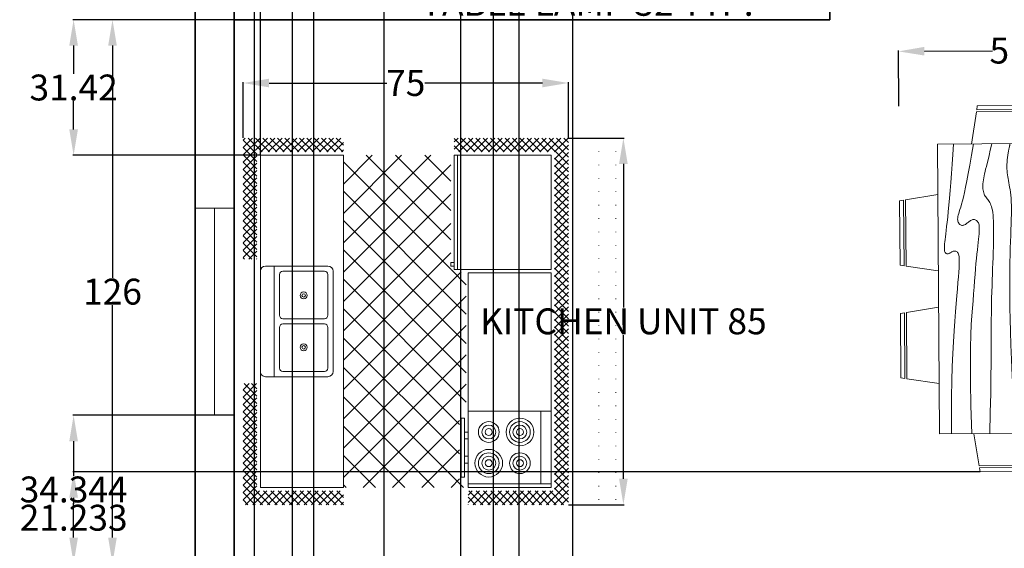
# Model space of a CAD drawing. Units: inches. Extents: x 351 to 774, y 111 to 703.
# Tile 2 of 6: x 380 to 608, y 342 to 464. Entities that reach past the tile are written whole.
import ezdxf

# ---------------------------------------------------------------- set-up
doc = ezdxf.new("R2010")
doc.units = ezdxf.units.IN
doc.header["$MEASUREMENT"] = 0
doc.linetypes.add('ACAD_ISO07W100', pattern=[3, 0, -3])
for name, color, linetype, lineweight in [('A-ANNO-DIMS', 2, 'Continuous', 18), ('A-EQPM-KTCH', 8, 'Continuous', 18), ('A-FURN', 8, 'Continuous', 18), ('A-GLAZ', 4, 'Continuous', 18), ('A-WALL', 7, 'Continuous', 35), ('A-WALL-OVHD', 7, 'ACAD_ISO07W100', 18)]:
    doc.layers.add(name, color=color, linetype=linetype, lineweight=lineweight)
doc.styles.get("Standard").update_dxf_attribs({"font": 'arial.ttf'})
doc.dimstyles.get("Standard").update_dxf_attribs({"dimtxt": 6, "dimasz": 6, "dimexe": 0.18, "dimexo": 0.0625, "dimgap": 0.09, "dimtad": 0, "dimtih": 1, "dimtoh": 1, "dimdec": 0, "dimzin": 0, "dimdsep": 46, "dimlunit": 3, "dimtxsty": 'Standard', "dimcen": 0.09, "dimadec": 0, "dimazin": 0, "dimtfac": 1, "dimtdec": 0, "dimtofl": 0, "dimtmove": 0, "dimatfit": 3, "dimfxl": 1, "dimtolj": 1, "dimtzin": 0, "dimarcsym": 0})

# ---------------------------------------------------------------- blocks, each defined once
blk = doc.blocks.new('Dining Set - 36 x 72 in.')
for p, q in [((-22, 27.5), (-22.1562, 26.50042)), ((-22, 27.5), (-6, 27.5)), ((-5.8437, 26.49966), (-6, 27.5)), ((6, 27.5), (5.8438, 26.50042)), ((6, 27.5), (22, 27.5)), ((22.1563, 26.49966), (22, 27.5)), ((-22.2343, 26.00059), (-23.4847, 17.99762)), ((-22.2304, 26), (-5.7608, 26)), ((-5.8416, 26.5), (-22.1534, 26.5)), ((-4.5152, 17.99762), (-5.7655, 25.99926)), ((5.7657, 26.00059), (4.5153, 17.99762)), ((5.7696, 26), (22.2392, 26)), ((22.1584, 26.5), (5.8466, 26.5)), ((23.4848, 17.99762), (22.2345, 25.99926)), ((36, 18), (-36, 18)), ((-36, 18), (-36, -18)), ((36, -18), (36, 18)), ((-45.5, 8), (-44.5004, 8.15617)), ((-45.5, 8), (-45.5, -8)), ((-44.5, -8.15843), (-44.5, 8.15338)), ((-44.0006, 8.23428), (-35.9976, 9.48474)), ((-44, 8.23041), (-44, -8.23915)), ((44.0006, 8.23428), (35.9976, 9.48474)), ((44, 8.23041), (44, -8.23915)), ((44.5, -8.15843), (44.5, 8.15338)), ((45.5, 8), (44.5005, 8.15617)), ((45.5, 8), (45.5, -8)), ((-44.4997, -8.15631), (-45.5, -8)), ((-35.9976, -9.48476), (-43.9993, -8.2345)), ((35.9976, -9.48476), (43.9993, -8.2345)), ((44.4997, -8.15631), (45.5, -8)), ((-36, -18), (36, -18)), ((-22.2343, -26.0006), (-23.4847, -17.99762)), ((-4.5152, -17.99762), (-5.7655, -25.99928)), ((5.7657, -26.0006), (4.5153, -17.99762)), ((23.4848, -17.99762), (22.2345, -25.99928)), ((-22.2304, -26), (-5.7608, -26)), ((-22, -27.5), (-22.1562, -26.50044)), ((-5.8416, -26.5), (-22.1534, -26.5)), ((-5.8437, -26.49967), (-6, -27.5)), ((5.7696, -26), (22.2392, -26)), ((6, -27.5), (5.8438, -26.50044)), ((22.1584, -26.5), (5.8466, -26.5)), ((22.1563, -26.49967), (22, -27.5)), ((-22, -27.5), (-6, -27.5)), ((6, -27.5), (22, -27.5))]:
    blk.add_line(p, q)
for points in [[(-36, 15), (-31.1772, 14.97754), (-26.8079, 14.91406), (-22.8538, 14.81543), (-19.276, 14.6875), (-16.0362, 14.53613), (-13.0957, 14.36718), (-10.4159, 14.18652), (-7.9583, 14), (-5.6904, 13.81315), (-3.6035, 13.63021), (-1.6954, 13.45508), (0.0365, 13.29166), (1.5945, 13.14388), (2.9811, 13.01562), (4.1988, 12.9108), (5.25, 12.83333), (6.1393, 12.78613), (6.8802, 12.76823), (7.4883, 12.77767), (7.9792, 12.8125), (8.3685, 12.87077), (8.6719, 12.95052), (8.9049, 13.0498), (9.0833, 13.16666), (9.2205, 13.29899), (9.3216, 13.44401), (9.3895, 13.59879), (9.4271, 13.76041), (9.4373, 13.92594), (9.4232, 14.09245), (9.3875, 14.257), (9.3333, 14.41666), (9.2638, 14.56917), (9.1836, 14.71484), (9.0975, 14.85465), (9.0104, 14.98958), (8.9272, 15.1206), (8.8529, 15.2487), (8.7922, 15.37483), (8.75, 15.5), (8.7305, 15.62467), (8.7344, 15.74739), (8.7617, 15.86621), (8.8125, 15.97916), (8.8867, 16.08431), (8.9844, 16.17968), (9.1055, 16.26334), (9.25, 16.33333), (9.4189, 16.38802), (9.6172, 16.42708), (9.8506, 16.45052), (10.125, 16.45833), (10.4463, 16.45052), (10.8203, 16.42708), (11.2529, 16.38802), (11.75, 16.33333), (12.3184, 16.26318), (12.9694, 16.17838), (13.7151, 16.07991), (14.5677, 15.96875), (15.5395, 15.84586), (16.6426, 15.71224), (17.8893, 15.56884), (19.2917, 15.41666), (20.859, 15.25667), (22.5879, 15.08984), (24.4721, 14.91715), (26.5052, 14.73958), (28.6809, 14.5581), (30.9929, 14.3737), (33.4347, 14.18733), (36, 14)], [(-36, 10), (-28.9766, 10.14274), (-23.1725, 10.20442), (-18.4241, 10.19775), (-14.5677, 10.13541), (-11.4399, 10.03011), (-8.877, 9.89453), (-6.7154, 9.74137), (-4.7917, 9.58333), (-2.9698, 9.43082), (-1.2246, 9.28515), (0.4415, 9.14534), (2.026, 9.01041), (3.5266, 8.87939), (4.9408, 8.7513), (6.266, 8.62516), (7.5, 8.5), (8.6411, 8.37549), (9.6914, 8.2539), (10.6538, 8.13818), (11.5312, 8.03125), (12.3267, 7.93603), (13.043, 7.85547), (13.6831, 7.79248), (14.25, 7.75), (14.7471, 7.7303), (15.1797, 7.73307), (15.5537, 7.75732), (15.875, 7.80208), (16.1494, 7.86637), (16.3828, 7.94922), (16.5811, 8.04964), (16.75, 8.16666), (16.8944, 8.29915), (17.0143, 8.44531), (17.1089, 8.60319), (17.1771, 8.77083), (17.218, 8.94629), (17.2305, 9.1276), (17.2137, 9.31282), (17.1667, 9.5), (17.0895, 9.6875), (16.987, 9.875), (16.8649, 10.0625), (16.7292, 10.25), (16.5856, 10.4375), (16.4401, 10.625), (16.2985, 10.8125), (16.1667, 11), (16.05, 11.18733), (15.9518, 11.3737), (15.8752, 11.5581), (15.8229, 11.73958), (15.798, 11.91715), (15.8034, 12.08984), (15.842, 12.25667), (15.9167, 12.41666), (16.0295, 12.56836), (16.1784, 12.70833), (16.3605, 12.83268), (16.5729, 12.9375), (16.8127, 13.01888), (17.0768, 13.07291), (17.3625, 13.0957), (17.6667, 13.08333), (17.9894, 13.03312), (18.3418, 12.94726), (18.7382, 12.82918), (19.1927, 12.68229), (19.7195, 12.51001), (20.3327, 12.31575), (21.0465, 12.10294), (21.875, 11.875), (22.8357, 11.63354), (23.959, 11.37304), (25.2786, 11.08618), (26.8282, 10.76562), (28.6414, 10.40405), (30.752, 9.99414), (33.1936, 9.52856), (36, 9)], [(-36, 5.5), (-30.7157, 5.3348), (-26.069, 5.20963), (-21.9946, 5.11767), (-18.4271, 5.05208), (-15.3009, 5.00602), (-12.5508, 4.97265), (-10.1112, 4.94515), (-7.9167, 4.91666), (-5.909, 4.88167), (-4.0586, 4.83984), (-2.3429, 4.79215), (-0.7396, 4.73958), (0.7739, 4.6831), (2.22, 4.6237), (3.6213, 4.56233), (5, 4.5), (6.373, 4.43782), (7.7344, 4.3776), (9.0723, 4.32129), (10.375, 4.27083), (11.6309, 4.22819), (12.8281, 4.19531), (13.9551, 4.17415), (15, 4.16666), (15.954, 4.17448), (16.819, 4.19791), (17.6001, 4.23698), (18.3021, 4.29166), (18.9299, 4.36198), (19.4883, 4.44791), (19.9823, 4.54948), (20.4167, 4.66666), (20.7969, 4.79899), (21.1302, 4.94401), (21.4245, 5.09879), (21.6875, 5.26041), (21.9271, 5.42594), (22.1511, 5.59245), (22.3672, 5.757), (22.5834, 5.91666), (22.8065, 6.06868), (23.0404, 6.21093), (23.2879, 6.34147), (23.5521, 6.45833), (23.8358, 6.55957), (24.142, 6.64323), (24.4735, 6.70735), (24.8334, 6.75), (25.2235, 6.76969), (25.642, 6.76692), (26.0858, 6.74267), (26.5521, 6.69791), (27.0379, 6.63362), (27.5404, 6.55078), (28.0565, 6.45036), (28.5834, 6.33333), (29.1242, 6.19987), (29.7071, 6.04687), (30.3661, 5.87044), (31.1354, 5.66666), (32.0493, 5.43164), (33.142, 5.16146), (34.4475, 4.85221), (36, 4.5)], [(-36, -1), (-30.7915, -0.6591), (-26.0195, -0.38216), (-21.6519, -0.16284), (-17.6563, 0.00521), (-14.0005, 0.12833), (-10.6523, 0.21289), (-7.5796, 0.26522), (-4.75, 0.29166), (-2.134, 0.29793), (0.2878, 0.28711), (2.5317, 0.26163), (4.6146, 0.22396), (6.5529, 0.17651), (8.3633, 0.12174), (10.0623, 0.06209), (11.6667, 0), (13.1899, -0.06201), (14.6341, -0.1211), (15.9982, -0.17432), (17.2813, -0.21875), (18.4823, -0.25147), (19.6003, -0.26953), (20.6343, -0.27002), (21.5834, -0.25), (22.4481, -0.20768), (23.2357, -0.14584), (23.9549, -0.06836), (24.6146, 0.02083), (25.2235, 0.11784), (25.7904, 0.21875), (26.3241, 0.31966), (26.8334, 0.41666), (27.3265, 0.50618), (27.8099, 0.58593), (28.2894, 0.65397), (28.7709, 0.70833), (29.2601, 0.74707), (29.763, 0.76823), (30.2855, 0.76985), (30.8334, 0.75), (31.4088, 0.70784), (31.9994, 0.64713), (32.589, 0.57275), (33.1615, 0.48958), (33.7008, 0.4025), (34.1908, 0.3164), (34.6153, 0.23616), (34.9584, 0.16666), (35.2099, 0.11165), (35.3848, 0.07031), (35.504, 0.04069), (35.5886, 0.02083), (35.6594, 0.00879), (35.7377, 0.0026), (35.8442, 0.00032), (36, 0)], [(-36, -6.5), (-27.1843, -6.31267), (-20.084, -6.1263), (-14.469, -5.9419), (-10.1094, -5.76042), (-6.7752, -5.58285), (-4.2363, -5.41016), (-2.2629, -5.24333), (-0.625, -5.08334), (0.8708, -4.93099), (2.2715, -4.78646), (3.5872, -4.64974), (4.8281, -4.52084), (6.0046, -4.39974), (7.127, -4.28646), (8.2053, -4.18099), (9.25, -4.08334), (10.2705, -3.99382), (11.2734, -3.91407), (12.2647, -3.84603), (13.25, -3.79167), (14.2354, -3.75293), (15.2266, -3.73177), (16.2295, -3.73015), (17.25, -3.75), (18.2912, -3.79248), (19.3451, -3.85547), (20.4009, -3.93604), (21.4479, -4.03125), (22.4754, -4.13819), (23.4727, -4.25391), (24.4289, -4.37549), (25.3334, -4.5), (26.1785, -4.62492), (26.9694, -4.74935), (27.7145, -4.87281), (28.4219, -4.99479), (29.1, -5.11483), (29.7572, -5.23242), (30.4016, -5.34709), (31.0417, -5.45834), (31.6837, -5.56437), (32.3262, -5.65821), (32.9658, -5.73153), (33.599, -5.77604), (34.2224, -5.78345), (34.8327, -5.74545), (35.4264, -5.65373), (36, -5.5)], [(-36, -10), (-26.4022, -9.81299), (-18.4675, -9.62891), (-11.9839, -9.45069), (-6.7396, -9.28125), (-2.5226, -9.12354), (0.8789, -8.98047), (3.6769, -8.85498), (6.0833, -8.75), (8.2767, -8.66765), (10.3021, -8.60677), (12.1712, -8.56543), (13.8958, -8.54167), (15.4876, -8.53353), (16.9583, -8.53907), (18.3197, -8.55632), (19.5834, -8.58334), (20.7616, -8.61841), (21.8685, -8.66081), (22.9188, -8.71004), (23.9271, -8.76563), (24.9081, -8.82707), (25.8763, -8.89388), (26.8465, -8.96558), (27.8334, -9.04167), (28.8474, -9.12118), (29.8828, -9.20117), (30.93, -9.27824), (31.9792, -9.34896), (33.0205, -9.40991), (34.0443, -9.45768), (35.0407, -9.48885), (36, -9.5)], [(-36, -14.5), (-30.0881, -14.33513), (-25.0332, -14.21224), (-20.7312, -14.12647), (-17.0781, -14.07292), (-13.97, -14.04671), (-11.3027, -14.04297), (-8.9724, -14.05681), (-6.875, -14.08334), (-4.9224, -14.11833), (-3.0905, -14.16016), (-1.3709, -14.20785), (0.2448, -14.26042), (1.7647, -14.3169), (3.1973, -14.3763), (4.5507, -14.43767), (5.8333, -14.5), (7.0554, -14.5621), (8.235, -14.62175), (9.3922, -14.67652), (10.5469, -14.72396), (11.7192, -14.76164), (12.929, -14.78711), (14.1965, -14.79794), (15.5417, -14.79167), (16.9933, -14.76424), (18.6152, -14.70508), (20.4804, -14.60197), (22.6615, -14.44271), (25.2312, -14.21509), (28.2624, -13.9069), (31.8277, -13.50594), (36, -13)]]:
    blk.add_lwpolyline(points)
blk = doc.blocks.new('Kitchen Layout - 7 x 8 ft')
for p, q in [((-5, 81.32), (2.68, 89)), ((-5, 83.44), (0.56, 89)), ((-5, 85.56), (-1.56, 89)), ((-5, 87.68), (-3.68, 89)), ((-1, 84.97), (-5, 88.97)), ((1.09, 85), (-2.91, 89)), ((3.21, 85), (-0.79, 89)), ((0.81, 85), (4.81, 89)), ((5.34, 85), (1.34, 89)), ((2.93, 85), (6.93, 89)), ((7.46, 85), (3.46, 89)), ((5.05, 85), (9.05, 89)), ((9.58, 85), (5.58, 89)), ((7.17, 85), (11.17, 89)), ((11.7, 85), (7.7, 89)), ((9.29, 85), (13.29, 89)), ((13.82, 85), (9.82, 89)), ((11.41, 85), (15.41, 89)), ((15.94, 85), (11.94, 89)), ((13.53, 85), (17.53, 89)), ((18.06, 85), (14.06, 89)), ((15.65, 85), (19.65, 89)), ((20.18, 85), (16.18, 89)), ((17.78, 85), (21.78, 89)), ((22.31, 85), (18.31, 89)), ((19.9, 85), (23.9, 89)), ((24.43, 85), (20.43, 89)), ((22.02, 85), (26.02, 89)), ((26.55, 85), (22.55, 89)), ((24.14, 85), (28.14, 89)), ((28.67, 85), (24.67, 89)), ((26.26, 85), (30.26, 89)), ((30.79, 85), (26.79, 89)), ((28.38, 85), (32.38, 89)), ((32.91, 85), (28.91, 89)), ((30.5, 85), (34.5, 89)), ((35.03, 85), (31.03, 89)), ((32.63, 85), (36.63, 89)), ((37.16, 85), (33.16, 89)), ((34.75, 85), (38.75, 89)), ((39.28, 85), (35.28, 89)), ((36.87, 85), (40.87, 89)), ((41.4, 85), (37.4, 89)), ((38.99, 85), (42.99, 89)), ((43.52, 85), (39.52, 89)), ((41.11, 85), (45.11, 89)), ((45.64, 85), (41.64, 89)), ((43.23, 85), (47.23, 89)), ((47.76, 85), (43.76, 89)), ((45.35, 85), (49.35, 89)), ((49.88, 85), (45.88, 89)), ((47.47, 85), (51.47, 89)), ((52, 85), (48, 89)), ((49.6, 85), (53.6, 89)), ((54.13, 85), (50.13, 89)), ((51.72, 85), (55.72, 89)), ((56.25, 85), (52.25, 89)), ((53.84, 85), (57.84, 89)), ((58.37, 85), (54.37, 89)), ((55.96, 85), (59.96, 89)), ((60.49, 85), (56.49, 89)), ((58.08, 85), (62.08, 89)), ((62.61, 85), (58.61, 89)), ((60.2, 85), (64.2, 89)), ((64.73, 85), (60.73, 89)), ((62.32, 85), (66.32, 89)), ((66.85, 85), (62.85, 89)), ((64.45, 85), (68.45, 89)), ((68.97, 85), (64.97, 89)), ((66.57, 85), (70.57, 89)), ((71.1, 85), (67.1, 89)), ((68.69, 85), (72.69, 89)), ((73.22, 85), (69.22, 89)), ((70.81, 85), (74.81, 89)), ((75.34, 85), (71.34, 89)), ((72.93, 85), (76.93, 89)), ((77.46, 85), (73.46, 89)), ((75.05, 85), (79.05, 89)), ((79.58, 85), (75.58, 89)), ((77.17, 85), (81.17, 89)), ((81.7, 85), (77.7, 89)), ((79.29, 85), (83.29, 89)), ((83.82, 85), (79.82, 89)), ((81.42, 85), (85.42, 89)), ((85.95, 85), (81.95, 89)), ((83.54, 85), (87.54, 89)), ((88.07, 85), (84.07, 89)), ((85.66, 85), (89.66, 89)), ((90.19, 85), (86.19, 89)), ((87.78, 85), (91.78, 89)), ((92.31, 85), (88.31, 89)), ((89.9, 85), (93.9, 89)), ((94.43, 85), (90.43, 89)), ((92.02, 85), (96.02, 89)), ((96.55, 85), (92.55, 89)), ((94.14, 85), (98.14, 89)), ((101, 82.67), (94.67, 89)), ((96.27, 85), (100.27, 89)), ((101, 84.79), (96.79, 89)), ((101, 86.92), (98.92, 89)), ((-1, 82.85), (-5, 86.85)), ((97, 83.61), (101, 87.61)), ((97, 81.49), (101, 85.49)), ((-1, 80.73), (-5, 84.73)), ((-5, 79.19), (-1, 83.19)), ((-1, 78.61), (-5, 82.61)), ((34, 84), (96, 84)), ((34, 60), (34, 84)), ((96, 84), (96, 60)), ((101, 80.55), (97, 84.55)), ((97, 79.37), (101, 83.37)), ((-5, 77.07), (-1, 81.07)), ((-1, 76.49), (-5, 80.49)), ((74, 81), (95, 81)), ((101, 78.43), (97, 82.43)), ((97, 77.25), (101, 81.25)), ((101, 76.31), (97, 80.31)), ((-5, 74.95), (-1, 78.95)), ((-1, 74.36), (-5, 78.36)), ((97, 75.13), (101, 79.13)), ((101, 74.19), (97, 78.19)), ((97, 73.01), (101, 77.01)), ((-5, 72.83), (-1, 76.83)), ((-1, 72.24), (-5, 76.24)), ((-5, 70.71), (-1, 74.71)), ((-1, 70.12), (-5, 74.12)), ((101, 72.07), (97, 76.07)), ((97, 70.89), (101, 74.89)), ((-5, 68.59), (-1, 72.59)), ((-1, 68), (-5, 72)), ((101, 69.95), (97, 73.95)), ((97, 68.76), (101, 72.76)), ((101, 67.82), (97, 71.82)), ((-5, 66.47), (-1, 70.47)), ((-1, 65.88), (-5, 69.88)), ((-5, 64.35), (-1, 68.35)), ((97, 66.64), (101, 70.64)), ((101, 65.7), (97, 69.7)), ((97, 64.52), (101, 68.52)), ((-1, 63.76), (-5, 67.76)), ((-5, 62.22), (-1, 66.22)), ((-1, 61.64), (-5, 65.64)), ((101, 63.58), (97, 67.58)), ((97, 62.4), (101, 66.4)), ((101, 61.46), (97, 65.46)), ((-5, 60.1), (-1, 64.1)), ((-1, 59.52), (-5, 63.52)), ((97, 60.28), (101, 64.28)), ((100.34, 60), (97, 63.34)), ((-5, 57.98), (-1, 61.98)), ((-1, 57.39), (-5, 61.39)), ((-4.86, 56), (-1, 59.86)), ((96, 60), (34, 60)), ((80, 60), (80, 59)), ((82, 59), (82, 60)), ((87, 59), (87, 60)), ((89, 60), (89, 59)), ((98.22, 60), (97, 61.22)), ((98.84, 60), (101, 62.16)), ((100.96, 60), (101, 60.04)), ((-1.73, 56), (-5, 59.27)), ((-3.85, 56), (-5, 57.15)), ((-2.74, 56), (-1, 57.74)), ((0, 57), (33, 57)), ((10.4, 24), (45.9, 59.5)), ((18.88, 24), (54.38, 59.5)), ((27.37, 24), (62.87, 59.5)), ((33.03, 55.11), (37.41, 59.5)), ((67.71, 24), (33.68, 58.04)), ((35.85, 24), (71.35, 59.5)), ((76.2, 24), (40.7, 59.5)), ((44.34, 24), (77.84, 57.5)), ((84.68, 24), (49.18, 59.5)), ((52.82, 24), (86.32, 57.5)), ((93.17, 24), (57.67, 59.5)), ((61.31, 24), (96, 58.69)), ((96, 29.65), (66.15, 59.5)), ((96, 38.14), (76.64, 57.5)), ((96, 46.63), (85.13, 57.5)), ((96, 55.11), (93.57, 57.54)), ((0, 30.57), (24.43, 55)), ((0, 39.06), (15.94, 55)), ((0, 47.54), (7.46, 55)), ((1.91, 24), (32.91, 55)), ((33.77, 24), (2.77, 55)), ((42.26, 24), (11.26, 55)), ((50.74, 24), (19.74, 55)), ((59.23, 24), (28.23, 55)), ((31, 55), (31, 56)), ((32, 55), (31, 55)), ((32, 56), (32, 55)), ((25.29, 24), (0, 49.29)), ((69.79, 24), (96, 50.21)), ((16.8, 24), (0, 40.8)), ((78.28, 24), (96, 41.72)), ((8.32, 24), (0, 32.32)), ((86.76, 24), (96, 33.24)), ((-5, 21.92), (-2.92, 24)), ((-5, 19.8), (-1, 23.8)), ((-1, 19.21), (-5, 23.21)), ((-1, 21.33), (-3.67, 24)), ((-1, 23.45), (-1.55, 24)), ((0, 24), (96, 24)), ((0, 0), (0, 24)), ((95.25, 24), (96, 24.75)), ((96, 24), (96, 0)), ((97, 22.1), (98.9, 24)), ((97, 19.97), (101, 23.97)), ((101, 19.03), (97, 23.03)), ((101, 21.16), (98.16, 24)), ((101, 23.28), (100.28, 24)), ((-5, 17.68), (-1, 21.68)), ((-1, 17.09), (-5, 21.09)), ((97, 17.85), (101, 21.85)), ((101, 16.91), (97, 20.91)), ((-5, 15.55), (-1, 19.55)), ((-1, 14.97), (-5, 18.97)), ((-5, 13.43), (-1, 17.43)), ((47.25, 6.5), (47.25, 18.5)), ((48.75, 18.5), (48.75, 6.5)), ((97, 15.73), (101, 19.73)), ((101, 14.79), (97, 18.79)), ((97, 13.61), (101, 17.61)), ((-1, 12.85), (-5, 16.85)), ((-5, 11.31), (-1, 15.31)), ((-1, 10.73), (-5, 14.73)), ((101, 12.67), (97, 16.67)), ((97, 11.49), (101, 15.49)), ((101, 10.55), (97, 14.55)), ((-5, 9.19), (-1, 13.19)), ((-1, 8.6), (-5, 12.6)), ((97, 9.37), (101, 13.37)), ((101, 8.43), (97, 12.43)), ((-5, 7.07), (-1, 11.07)), ((-1, 6.48), (-5, 10.48)), ((-5, 4.95), (-1, 8.95)), ((97, 7.25), (101, 11.25)), ((101, 6.31), (97, 10.31)), ((97, 5.12), (101, 9.12)), ((-1, 4.36), (-5, 8.36)), ((-5, 2.83), (-1, 6.83)), ((-1, 2.24), (-5, 6.24)), ((101, 4.18), (97, 8.18)), ((97, 3), (101, 7)), ((101, 2.06), (97, 6.06)), ((-5, 0.71), (-1, 4.71)), ((-1, 0.12), (-5, 4.12)), ((64, 4), (32, 4)), ((97, 0.88), (101, 4.88)), ((101, -0.06), (97, 3.94)), ((-5, -1.42), (-1, 2.58)), ((2, -5), (-5, 2)), ((-5, -3.54), (-1, 0.46)), ((96, 0), (0, 0)), ((93.24, -5), (101, 2.76)), ((95.36, -5), (101, 0.64)), ((101, -2.18), (97, 1.82)), ((-0.12, -5), (-5, -0.12)), ((-2.25, -5), (-5, -2.25)), ((-4.34, -5), (-0.34, -1)), ((-2.22, -5), (1.78, -1)), ((-0.1, -5), (3.9, -1)), ((4.12, -5), (0.12, -1)), ((2.02, -5), (6.02, -1)), ((6.24, -5), (2.24, -1)), ((4.14, -5), (8.14, -1)), ((8.36, -5), (4.36, -1)), ((6.27, -5), (10.27, -1)), ((10.48, -5), (6.48, -1)), ((8.39, -5), (12.39, -1)), ((12.6, -5), (8.6, -1)), ((10.51, -5), (14.51, -1)), ((14.73, -5), (10.73, -1)), ((12.63, -5), (16.63, -1)), ((16.85, -5), (12.85, -1)), ((14.75, -5), (18.75, -1)), ((18.97, -5), (14.97, -1)), ((16.87, -5), (20.87, -1)), ((21.09, -5), (17.09, -1)), ((18.99, -5), (22.99, -1)), ((23.21, -5), (19.21, -1)), ((21.11, -5), (25.11, -1)), ((25.33, -5), (21.33, -1)), ((23.24, -5), (27.24, -1)), ((27.45, -5), (23.45, -1)), ((25.36, -5), (29.36, -1)), ((29.57, -5), (25.57, -1)), ((27.48, -5), (30, -2.48)), ((30, -3.3), (27.7, -1)), ((30, -1.18), (29.82, -1)), ((66, -2.54), (67.54, -1)), ((66, -4.66), (69.66, -1)), ((69.88, -5), (66, -1.12)), ((67.78, -5), (71.78, -1)), ((72, -5), (68, -1)), ((69.9, -5), (73.9, -1)), ((74.12, -5), (70.12, -1)), ((72.03, -5), (76.03, -1)), ((76.24, -5), (72.24, -1)), ((74.15, -5), (78.15, -1)), ((78.36, -5), (74.36, -1)), ((76.27, -5), (80.27, -1)), ((80.49, -5), (76.49, -1)), ((78.39, -5), (82.39, -1)), ((82.61, -5), (78.61, -1)), ((80.51, -5), (84.51, -1)), ((84.73, -5), (80.73, -1)), ((82.63, -5), (86.63, -1)), ((86.85, -5), (82.85, -1)), ((84.75, -5), (88.75, -1)), ((88.97, -5), (84.97, -1)), ((86.88, -5), (90.88, -1)), ((91.09, -5), (87.09, -1)), ((89, -5), (93, -1)), ((93.21, -5), (89.21, -1)), ((91.12, -5), (95.12, -1)), ((95.34, -5), (91.34, -1)), ((97.46, -5), (93.46, -1)), ((99.58, -5), (95.58, -1)), ((101, -4.3), (97, -0.3)), ((97.48, -5), (101, -1.48)), ((-4.37, -5), (-5, -4.37)), ((29.6, -5), (30, -4.6)), ((67.76, -5), (66, -3.24)), ((99.6, -5), (101, -3.6))]:
    blk.add_line(p, q)
for points in [[(0, 56), (0, 84), (33, 84), (33, 56)], [(74, 60), (74, 84), (95, 84), (95, 60)], [(76, 58), (76, 59), (93, 59), (93, 58)]]:
    blk.add_lwpolyline(points, close=True)
for points in [[(33.5, 21), (62.5, 21)], [(32, 1.5), (32, 19.5)], [(33.5, 6.5), (33.5, 18.5)], [(34.5, 19.5), (46.25, 19.5)], [(49.75, 19.5), (61.5, 19.5)], [(62.5, 18.5), (62.5, 6.5)], [(64, 19.5), (64, 1.5)], [(46.25, 5.5), (34.5, 5.5)], [(61.5, 5.5), (49.75, 5.5)], [(62.5, 0), (33.5, 0)]]:
    blk.add_lwpolyline(points)
for centre, radius in [((80, 75), 4), ((80, 75), 3), ((80, 75), 2), ((89, 75), 3), ((89, 75), 2), ((80, 75), 1), ((89, 75), 1), ((80, 66), 3), ((89, 66), 4), ((89, 66), 3), ((80, 66), 2), ((80, 66), 1), ((89, 66), 2), ((89, 66), 1), ((40.5, 12.5), 1), ((40.5, 12.5), 0.5), ((55.5, 12.5), 1), ((55.5, 12.5), 0.5)]:
    blk.add_circle(centre, radius)
for centre, radius, start, end in [((33.5, 19.5), 1.5, 90, 180), ((62.5, 19.5), 1.5, 0, 90), ((34.5, 18.5), 1, 90, 180), ((46.25, 18.5), 1, 0, 90), ((49.75, 18.5), 1, 90, 180), ((61.5, 18.5), 1, 0, 90), ((34.5, 6.5), 1, 180, 270), ((46.25, 6.5), 1, 270, 0), ((49.75, 6.5), 1, 180, 270), ((61.5, 6.5), 1, 270, 0), ((33.5, 1.5), 1.5, 180, 270), ((62.5, 1.5), 1.5, 270, 0)]:
    blk.add_arc(centre, radius, start, end)
blk = doc.blocks.new('WIN-48IN-9IN-WALL')
blk.add_line((4.5, 48), (4.5, 0))
blk.add_lwpolyline([(0, 0), (9, 0), (9, 48), (0, 48)], close=True)
blk = doc.blocks.new('*D28')
at = {"layer": 'A-ANNO-DIMS', "color": 0, "lineweight": -2, "transparency": 16777216}
for p, q in [((432.23, 472.86), (432.23, 467.97)), ((464.06, 472.86), (464.06, 467.97)), ((438.23, 468.15), (458.06, 468.15)), ((464.06, 468.15), (470.06, 468.15))]:
    blk.add_line(p, q, dxfattribs=at)
at = {"layer": 'A-ANNO-DIMS', "color": 0, "transparency": 16777216}
for points in [[(438.23, 469.15), (438.23, 467.15), (432.23, 468.15)], [(458.06, 469.15), (458.06, 467.15), (464.06, 468.15)]]:
    blk.add_solid(points, dxfattribs=at)
at = {"layer": 'Defpoints', "color": 0, "transparency": 16777216}
for p in [(432.23, 472.92), (464.06, 472.92), (464.06, 468.15)]:
    blk.add_point(p, dxfattribs=at)
at = {"layer": 'A-ANNO-DIMS', "color": 0, "transparency": 16777216, "insert": (511.85, 468.15), "char_height": 6, "attachment_point": 5}
blk.add_mtext('\\A1;TABLE LAMP 32 TYP.', dxfattribs=at)
blk = doc.blocks.new('*D37')
at = {"layer": 'A-ANNO-DIMS', "color": 0, "lineweight": -2, "transparency": 16777216}
for p, q in [((584.02, 444.23), (583.93, 457.08)), ((589.93, 456.94), (605.75, 457.06)), ((629.2, 457.23), (613.37, 457.11)), ((635.29, 444.61), (635.2, 457.45))]:
    blk.add_line(p, q, dxfattribs=at)
at = {"layer": 'A-ANNO-DIMS', "color": 0, "transparency": 16777216}
for points in [[(589.92, 457.94), (589.93, 455.94), (583.93, 456.9)], [(629.19, 458.23), (629.21, 456.23), (635.2, 457.27)]]:
    blk.add_solid(points, dxfattribs=at)
at = {"layer": 'Defpoints', "color": 0, "transparency": 16777216}
for p in [(583.93, 456.9), (584.02, 444.17), (635.29, 444.55)]:
    blk.add_point(p, dxfattribs=at)
at = {"layer": 'A-ANNO-DIMS', "color": 0, "transparency": 16777216, "insert": (609.56, 457.08), "char_height": 6, "attachment_point": 5}
blk.add_mtext('\\A1;51', dxfattribs=at)
blk = doc.blocks.new('*D44')
at = {"layer": 'A-ANNO-DIMS', "color": 0, "lineweight": -2, "transparency": 16777216}
for p, q in [((507.54, 436.83), (520.4, 436.83)), ((520.22, 430.83), (520.22, 397.55)), ((520.22, 357.88), (520.22, 391.16)), ((507.54, 351.88), (520.4, 351.88))]:
    blk.add_line(p, q, dxfattribs=at)
at = {"layer": 'A-ANNO-DIMS', "color": 0, "transparency": 16777216}
for points in [[(519.22, 430.83), (521.22, 430.83), (520.22, 436.83)], [(519.22, 357.88), (521.22, 357.88), (520.22, 351.88)]]:
    blk.add_solid(points, dxfattribs=at)
at = {"layer": 'Defpoints', "color": 0, "transparency": 16777216}
for p in [(507.48, 436.83), (507.48, 351.88), (520.22, 351.88)]:
    blk.add_point(p, dxfattribs=at)
at = {"layer": 'A-ANNO-DIMS', "color": 0, "transparency": 16777216, "insert": (520.22, 394.36), "char_height": 6, "attachment_point": 5}
blk.add_mtext('\\A1;KITCHEN UNIT 85', dxfattribs=at)
blk = doc.blocks.new('*D45')
at = {"layer": 'A-ANNO-DIMS', "color": 0, "lineweight": -2, "transparency": 16777216}
for p, q in [((432.15, 436.89), (432.15, 449.75)), ((438.15, 449.57), (465.43, 449.57)), ((501.48, 449.57), (474.2, 449.57)), ((507.48, 436.89), (507.48, 449.75))]:
    blk.add_line(p, q, dxfattribs=at)
at = {"layer": 'A-ANNO-DIMS', "color": 0, "transparency": 16777216}
for points in [[(438.15, 450.57), (438.15, 448.57), (432.15, 449.57)], [(501.48, 450.57), (501.48, 448.57), (507.48, 449.57)]]:
    blk.add_solid(points, dxfattribs=at)
at = {"layer": 'Defpoints', "color": 0, "transparency": 16777216}
for p in [(507.48, 449.57), (432.15, 436.83), (507.48, 436.83)]:
    blk.add_point(p, dxfattribs=at)
at = {"layer": 'A-ANNO-DIMS', "color": 0, "transparency": 16777216, "insert": (469.81, 449.57), "char_height": 6, "attachment_point": 5}
blk.add_mtext('\\A1;75', dxfattribs=at)
blk = doc.blocks.new('*D50')
at = {"layer": 'A-ANNO-DIMS', "color": 0, "lineweight": -2, "transparency": 16777216}
for p, q in [((421.04, 671.18), (421.04, 114.91)), ((443.48, 671.18), (443.48, 114.91)), ((427.04, 115.09), (437.48, 115.09)), ((443.48, 115.09), (449.48, 115.09))]:
    blk.add_line(p, q, dxfattribs=at)
at = {"layer": 'A-ANNO-DIMS', "color": 0, "transparency": 16777216}
for points in [[(427.04, 116.09), (427.04, 114.09), (421.04, 115.09)], [(437.48, 116.09), (437.48, 114.09), (443.48, 115.09)]]:
    blk.add_solid(points, dxfattribs=at)
at = {"layer": 'Defpoints', "color": 0, "transparency": 16777216}
for p in [(421.04, 671.24), (443.48, 671.24), (443.48, 115.09)]:
    blk.add_point(p, dxfattribs=at)
at = {"layer": 'A-ANNO-DIMS', "color": 0, "transparency": 16777216, "insert": (462.06, 115.09), "char_height": 6, "attachment_point": 5}
blk.add_mtext('\\A1;22.434', dxfattribs=at)
blk = doc.blocks.new('*D55')
at = {"layer": 'A-ANNO-DIMS', "color": 0, "lineweight": -2, "transparency": 16777216}
for p, q in [((429.98, 372.59), (392.71, 372.59)), ((392.89, 366.59), (392.89, 358.57)), ((392.89, 344.24), (392.89, 352.26)), ((429.98, 338.24), (392.71, 338.24))]:
    blk.add_line(p, q, dxfattribs=at)
at = {"layer": 'A-ANNO-DIMS', "color": 0, "transparency": 16777216}
for points in [[(391.89, 366.59), (393.89, 366.59), (392.89, 372.59)], [(391.89, 344.24), (393.89, 344.24), (392.89, 338.24)]]:
    blk.add_solid(points, dxfattribs=at)
at = {"layer": 'Defpoints', "color": 0, "transparency": 16777216}
for p in [(392.89, 372.59), (430.04, 372.59), (430.04, 338.24)]:
    blk.add_point(p, dxfattribs=at)
at = {"layer": 'A-ANNO-DIMS', "color": 0, "transparency": 16777216, "insert": (392.89, 355.41), "char_height": 6, "attachment_point": 5}
blk.add_mtext('\\A1;34.344', dxfattribs=at)
blk = doc.blocks.new('*D56')
at = {"layer": 'A-ANNO-DIMS', "color": 0, "lineweight": -2, "transparency": 16777216}
for p, q in [((429.98, 464.24), (401.71, 464.24)), ((401.89, 458.24), (401.89, 404.4)), ((401.89, 344.24), (401.89, 398.09)), ((429.98, 338.24), (401.71, 338.24))]:
    blk.add_line(p, q, dxfattribs=at)
at = {"layer": 'A-ANNO-DIMS', "color": 0, "transparency": 16777216}
for points in [[(400.89, 458.24), (402.89, 458.24), (401.89, 464.24)], [(400.89, 344.24), (402.89, 344.24), (401.89, 338.24)]]:
    blk.add_solid(points, dxfattribs=at)
at = {"layer": 'Defpoints', "color": 0, "transparency": 16777216}
for p in [(401.89, 464.24), (430.04, 464.24), (430.04, 338.24)]:
    blk.add_point(p, dxfattribs=at)
at = {"layer": 'A-ANNO-DIMS', "color": 0, "transparency": 16777216, "insert": (401.89, 401.24), "char_height": 6, "attachment_point": 5}
blk.add_mtext('\\A1;126', dxfattribs=at)
blk = doc.blocks.new('*D70')
at = {"layer": 'A-ANNO-DIMS', "color": 0, "lineweight": -2, "transparency": 16777216}
for p, q in [((430.04, 614.18), (430.04, 114.91)), ((434.71, 614.18), (434.71, 114.91)), ((424.04, 115.09), (418.04, 115.09)), ((440.71, 115.09), (446.71, 115.09))]:
    blk.add_line(p, q, dxfattribs=at)
at = {"layer": 'A-ANNO-DIMS', "color": 0, "transparency": 16777216}
for points in [[(424.04, 116.09), (424.04, 114.09), (430.04, 115.09)], [(440.71, 116.09), (440.71, 114.09), (434.71, 115.09)]]:
    blk.add_solid(points, dxfattribs=at)
at = {"layer": 'Defpoints', "color": 0, "transparency": 16777216}
for p in [(430.04, 614.24), (434.71, 614.24), (434.71, 115.09)]:
    blk.add_point(p, dxfattribs=at)
at = {"layer": 'A-ANNO-DIMS', "color": 0, "transparency": 16777216, "insert": (457.05, 115.09), "char_height": 6, "attachment_point": 5}
blk.add_mtext('\\A1;4.669', dxfattribs=at)
blk = doc.blocks.new('*D71')
at = {"layer": 'A-ANNO-DIMS', "color": 0, "lineweight": -2, "transparency": 16777216}
for p, q in [((434.71, 614.18), (434.71, 114.91)), ((464.71, 614.18), (464.71, 114.91)), ((440.71, 115.09), (445.34, 115.09)), ((458.71, 115.09), (454.09, 115.09))]:
    blk.add_line(p, q, dxfattribs=at)
at = {"layer": 'A-ANNO-DIMS', "color": 0, "transparency": 16777216}
for points in [[(440.71, 116.09), (440.71, 114.09), (434.71, 115.09)], [(458.71, 116.09), (458.71, 114.09), (464.71, 115.09)]]:
    blk.add_solid(points, dxfattribs=at)
at = {"layer": 'Defpoints', "color": 0, "transparency": 16777216}
for p in [(434.71, 614.24), (464.71, 614.24), (464.71, 115.09)]:
    blk.add_point(p, dxfattribs=at)
at = {"layer": 'A-ANNO-DIMS', "color": 0, "transparency": 16777216, "insert": (449.71, 115.09), "char_height": 6, "attachment_point": 5}
blk.add_mtext('\\A1;30', dxfattribs=at)
blk = doc.blocks.new('*D91')
at = {"layer": 'A-ANNO-DIMS', "color": 0, "lineweight": -2, "transparency": 16777216}
for p, q in [((496.04, 614.18), (496.04, 114.91)), ((508.41, 614.18), (508.41, 114.91)), ((502.04, 115.09), (502.41, 115.09)), ((508.41, 115.09), (514.41, 115.09))]:
    blk.add_line(p, q, dxfattribs=at)
at = {"layer": 'A-ANNO-DIMS', "color": 0, "transparency": 16777216}
for points in [[(502.04, 116.09), (502.04, 114.09), (496.04, 115.09)], [(502.41, 116.09), (502.41, 114.09), (508.41, 115.09)]]:
    blk.add_solid(points, dxfattribs=at)
at = {"layer": 'Defpoints', "color": 0, "transparency": 16777216}
for p in [(496.04, 614.24), (508.41, 614.24), (508.41, 115.09)]:
    blk.add_point(p, dxfattribs=at)
at = {"layer": 'A-ANNO-DIMS', "color": 0, "transparency": 16777216, "insert": (526.65, 115.09), "char_height": 6, "attachment_point": 5}
blk.add_mtext('\\A1;12.372', dxfattribs=at)
blk = doc.blocks.new('*D94')
at = {"layer": 'A-ANNO-DIMS', "color": 0, "lineweight": -2, "transparency": 16777216}
for p, q in [((424.04, 699.39), (418.04, 699.39)), ((430.04, 464.3), (430.04, 699.57)), ((436.15, 432.88), (436.15, 699.57)), ((442.15, 699.39), (448.15, 699.39))]:
    blk.add_line(p, q, dxfattribs=at)
at = {"layer": 'A-ANNO-DIMS', "color": 0, "transparency": 16777216}
for points in [[(424.04, 700.39), (424.04, 698.39), (430.04, 699.39)], [(442.15, 700.39), (442.15, 698.39), (436.15, 699.39)]]:
    blk.add_solid(points, dxfattribs=at)
at = {"layer": 'Defpoints', "color": 0, "transparency": 16777216}
for p in [(430.04, 699.39), (430.04, 464.24), (436.15, 432.82)]:
    blk.add_point(p, dxfattribs=at)
at = {"layer": 'A-ANNO-DIMS', "color": 0, "transparency": 16777216, "insert": (410.72, 699.39), "char_height": 6, "attachment_point": 5}
blk.add_mtext('\\A1;6.11', dxfattribs=at)
blk = doc.blocks.new('*D95')
at = {"layer": 'A-ANNO-DIMS', "color": 0, "lineweight": -2, "transparency": 16777216}
for p, q in [((429.98, 464.24), (392.71, 464.24)), ((392.89, 458.24), (392.89, 451.69)), ((392.89, 438.82), (392.89, 445.38)), ((436.09, 432.82), (392.71, 432.82))]:
    blk.add_line(p, q, dxfattribs=at)
at = {"layer": 'A-ANNO-DIMS', "color": 0, "transparency": 16777216}
for points in [[(391.89, 458.24), (393.89, 458.24), (392.89, 464.24)], [(391.89, 438.82), (393.89, 438.82), (392.89, 432.82)]]:
    blk.add_solid(points, dxfattribs=at)
at = {"layer": 'Defpoints', "color": 0, "transparency": 16777216}
for p in [(430.04, 464.24), (392.89, 432.82), (436.15, 432.82)]:
    blk.add_point(p, dxfattribs=at)
at = {"layer": 'A-ANNO-DIMS', "color": 0, "transparency": 16777216, "insert": (392.89, 448.53), "char_height": 6, "attachment_point": 5}
blk.add_mtext('\\A1;31.42', dxfattribs=at)
blk = doc.blocks.new('*D97')
at = {"layer": 'A-ANNO-DIMS', "color": 0, "lineweight": -2, "transparency": 16777216}
for p, q in [((602.76, 359.47), (392.71, 359.47)), ((392.89, 353.47), (392.89, 352.01)), ((392.89, 344.24), (392.89, 345.7)), ((608.38, 338.24), (392.71, 338.24))]:
    blk.add_line(p, q, dxfattribs=at)
at = {"layer": 'A-ANNO-DIMS', "color": 0, "transparency": 16777216}
for points in [[(391.89, 353.47), (393.89, 353.47), (392.89, 359.47)], [(391.89, 344.24), (393.89, 344.24), (392.89, 338.24)]]:
    blk.add_solid(points, dxfattribs=at)
at = {"layer": 'Defpoints', "color": 0, "transparency": 16777216}
for p in [(602.82, 359.47), (392.89, 338.24), (608.45, 338.24)]:
    blk.add_point(p, dxfattribs=at)
at = {"layer": 'A-ANNO-DIMS', "color": 0, "transparency": 16777216, "insert": (392.89, 348.86), "char_height": 6, "attachment_point": 5}
blk.add_mtext('\\A1;21.233', dxfattribs=at)
blk = doc.blocks.new('*D99')
at = {"layer": 'A-ANNO-DIMS', "color": 0, "lineweight": -2, "transparency": 16777216}
for p, q in [((482.51, 629.76), (482.51, 114.91)), ((490.04, 614.18), (490.04, 114.91)), ((476.51, 115.09), (470.51, 115.09)), ((496.04, 115.09), (502.04, 115.09))]:
    blk.add_line(p, q, dxfattribs=at)
at = {"layer": 'A-ANNO-DIMS', "color": 0, "transparency": 16777216}
for points in [[(476.51, 116.09), (476.51, 114.09), (482.51, 115.09)], [(496.04, 116.09), (496.04, 114.09), (490.04, 115.09)]]:
    blk.add_solid(points, dxfattribs=at)
at = {"layer": 'Defpoints', "color": 0, "transparency": 16777216}
for p in [(482.51, 629.82), (490.04, 614.24), (490.04, 115.09)]:
    blk.add_point(p, dxfattribs=at)
at = {"layer": 'A-ANNO-DIMS', "color": 0, "transparency": 16777216, "insert": (512.24, 115.09), "char_height": 6, "attachment_point": 5}
blk.add_mtext('\\A1;7.528', dxfattribs=at)
blk = doc.blocks.new('*D100')
at = {"layer": 'A-ANNO-DIMS', "color": 0, "lineweight": -2, "transparency": 16777216}
for p, q in [((430.04, 662.18), (430.04, 114.91)), ((448.42, 661.61), (448.42, 114.91)), ((430.04, 115.09), (424.04, 115.09)), ((442.42, 115.09), (436.04, 115.09))]:
    blk.add_line(p, q, dxfattribs=at)
at = {"layer": 'A-ANNO-DIMS', "color": 0, "transparency": 16777216}
for points in [[(436.04, 116.09), (436.04, 114.09), (430.04, 115.09)], [(442.42, 116.09), (442.42, 114.09), (448.42, 115.09)]]:
    blk.add_solid(points, dxfattribs=at)
at = {"layer": 'Defpoints', "color": 0, "transparency": 16777216}
for p in [(430.04, 662.24), (448.42, 661.68), (430.04, 115.09)]:
    blk.add_point(p, dxfattribs=at)
at = {"layer": 'A-ANNO-DIMS', "color": 0, "transparency": 16777216, "insert": (411.78, 115.09), "char_height": 6, "attachment_point": 5}
blk.add_mtext('\\A1;18.373', dxfattribs=at)

msp = doc.modelspace()

# ---------------------------------------------------------------- linework, layer by layer
at = {"layer": 'A-WALL'}
for p, q in [((568.043, 470.2421), (568.043, 464.2421)), ((430.043, 464.2421), (568.043, 464.2421)), ((430.043, 338.2421), (430.043, 464.2421))]:
    msp.add_line(p, q, dxfattribs=at)
msp.add_lwpolyline([(436.7781, 143.2421), (421.043, 143.2421), (421.043, 671.2421), (733.043, 671.2421), (733.043, 143.2421), (562.043, 143.2421)], dxfattribs=at)
at = {"layer": 'A-WALL-OVHD'}
for p, q in [((514.5, 436.8284), (514.5, 351.8818)), ((514.5, 436.8284), (518.5, 436.8284)), ((518.5, 436.8284), (518.5, 351.8818)), ((514.5, 351.8818), (514.6351, 351.8818)), ((514.6351, 351.8818), (518.5, 351.8818))]:
    msp.add_line(p, q, dxfattribs=at)

# ---------------------------------------------------------------- block references
at = {"layer": 'A-EQPM-KTCH', "xscale": 0.8013826619265847, "yscale": 0.8013826619265847, "zscale": 0.8013826619265847, "rotation": 270}
msp.add_blockref('Kitchen Layout - 7 x 8 ft', (436.1529, 432.8215), dxfattribs=at)
at = {"layer": 'A-FURN', "xscale": 0.9322251862135446, "yscale": 0.9322251862135446, "zscale": 0.9322251862135446, "rotation": 90.42208138352696}
msp.add_blockref('Dining Set - 36 x 72 in.', (609.9687, 401.9447), dxfattribs=at)
at = {"layer": 'A-GLAZ'}
msp.add_blockref('WIN-48IN-9IN-WALL', (421.043, 372.5866), dxfattribs=at)

# ---------------------------------------------------------------- dimensions: what is measured, and where the dimension line sits
at = {"layer": 'A-ANNO-DIMS'}
for base, p1, p2, override, picture, middle in [((430.043, 699.3921), (436.1529, 432.8215), (430.043, 464.2421), {"dimdec": 2, "dimlfac": 1, "dimrnd": 0, "dimzin": 0, "dimdsep": 46, "dimlunit": 2}, '*D94', (410.7231, 699.3921)), ((443.4772, 115.0921), (421.043, 671.2421), (443.4772, 671.2421), {"dimdec": 3, "dimlfac": 1, "dimrnd": 0, "dimzin": 0, "dimdsep": 46, "dimlunit": 2}, '*D50', (462.0604, 115.0921)), ((430.043, 115.0921), (448.416, 661.6763), (430.043, 662.2421), {"dimdec": 3, "dimlfac": 1, "dimrnd": 0, "dimzin": 0, "dimdsep": 46, "dimlunit": 2}, '*D100', (411.7811, 115.0921)), ((490.043, 115.0921), (482.5147, 629.8184), (490.043, 614.2421), {"dimdec": 3, "dimlfac": 1, "dimrnd": 0, "dimzin": 0, "dimdsep": 46, "dimlunit": 2}, '*D99', (512.2381, 115.0921)), ((434.7119, 115.0921), (430.043, 614.2421), (434.7119, 614.2421), {"dimdec": 3, "dimlfac": 1, "dimrnd": 0, "dimzin": 0, "dimdsep": 46, "dimlunit": 2}, '*D70', (457.0522, 115.0921)), ((464.7119, 115.0921), (434.7119, 614.2421), (464.7119, 614.2421), {"dimdec": 0, "dimlfac": 1, "dimrnd": 0, "dimzin": 0, "dimdsep": 46, "dimlunit": 2}, '*D71', (449.7119, 115.0921)), ((508.4146, 115.0921), (496.043, 614.2421), (508.4146, 614.2421), {"dimdec": 3, "dimlfac": 1, "dimrnd": 0, "dimzin": 0, "dimdsep": 46, "dimlunit": 2}, '*D91', (526.6458, 115.0921)), ((507.476, 449.5704), (432.146, 436.8284), (507.476, 436.8284), {"dimdec": 0, "dimlfac": 1, "dimrnd": 0, "dimzin": 0, "dimdsep": 46, "dimlunit": 2}, '*D45', (469.811, 449.5704))]:
    dim = msp.add_linear_dim(base=base, p1=p1, p2=p2, dimstyle='Standard', override=override, dxfattribs=at)
    dim.commit()
    dim.dimension.update_dxf_attribs({"geometry": picture, "text_midpoint": middle})
dim = msp.add_linear_dim(base=(464.0615, 468.1493), p1=(432.2338, 472.9235), p2=(464.0615, 472.9235), text='TABLE LAMP <> TYP.', dimstyle='Standard', override={"dimdec": 0, "dimlfac": 1, "dimrnd": 0, "dimzin": 0, "dimdsep": 46, "dimlunit": 2}, dxfattribs=at)
dim.commit()
dim.dimension.update_dxf_attribs({"geometry": '*D28', "text_midpoint": (511.8486, 468.1493)})
for base, p1, p2, angle, override, picture, middle in [((392.893, 432.8215), (430.043, 464.2421), (436.1529, 432.8215), 90, {"dimdec": 2, "dimlfac": 1, "dimrnd": 0, "dimzin": 0, "dimdsep": 46, "dimlunit": 2}, '*D95', (392.893, 448.5318)), ((401.893, 464.2421), (430.043, 338.2421), (430.043, 464.2421), 90, {"dimdec": 0, "dimlfac": 1, "dimrnd": 0, "dimzin": 0, "dimdsep": 46, "dimlunit": 2}, '*D56', (401.893, 401.2421)), ((583.927, 456.8954), (635.2917, 444.5486), (584.0207, 444.1709), 180.422081, {"dimdec": 0, "dimlfac": 1, "dimrnd": 0, "dimzin": 0, "dimdsep": 46, "dimlunit": 2}, '*D37', (609.5625, 457.0843)), ((392.89303, 372.58657), (430.04303, 338.24208), (430.04303, 372.58657), 90, {"dimdec": 3, "dimlfac": 1, "dimrnd": 0, "dimzin": 0, "dimdsep": 46, "dimlunit": 2}, '*D55', (392.89303, 355.41432)), ((392.89303, 338.24208), (602.82353, 359.47464), (608.44737, 338.24208), 90, {"dimdec": 3, "dimlfac": 1, "dimrnd": 0, "dimzin": 0, "dimdsep": 46, "dimlunit": 2}, '*D97', (392.89303, 348.85836))]:
    dim = msp.add_linear_dim(base=base, p1=p1, p2=p2, angle=angle, dimstyle='Standard', override=override, dxfattribs=at)
    dim.commit()
    dim.dimension.update_dxf_attribs({"geometry": picture, "text_midpoint": middle})
dim = msp.add_linear_dim(base=(520.218, 351.8818), p1=(507.476, 436.8284), p2=(507.476, 351.8818), angle=270, text='KITCHEN UNIT <>', dimstyle='Standard', override={"dimdec": 0, "dimlfac": 1, "dimrnd": 0, "dimzin": 0, "dimdsep": 46, "dimlunit": 2}, dxfattribs=at)
dim.commit()
dim.dimension.update_dxf_attribs({"geometry": '*D44', "text_midpoint": (520.218, 394.3551)})

doc.saveas('drawing.dxf')
